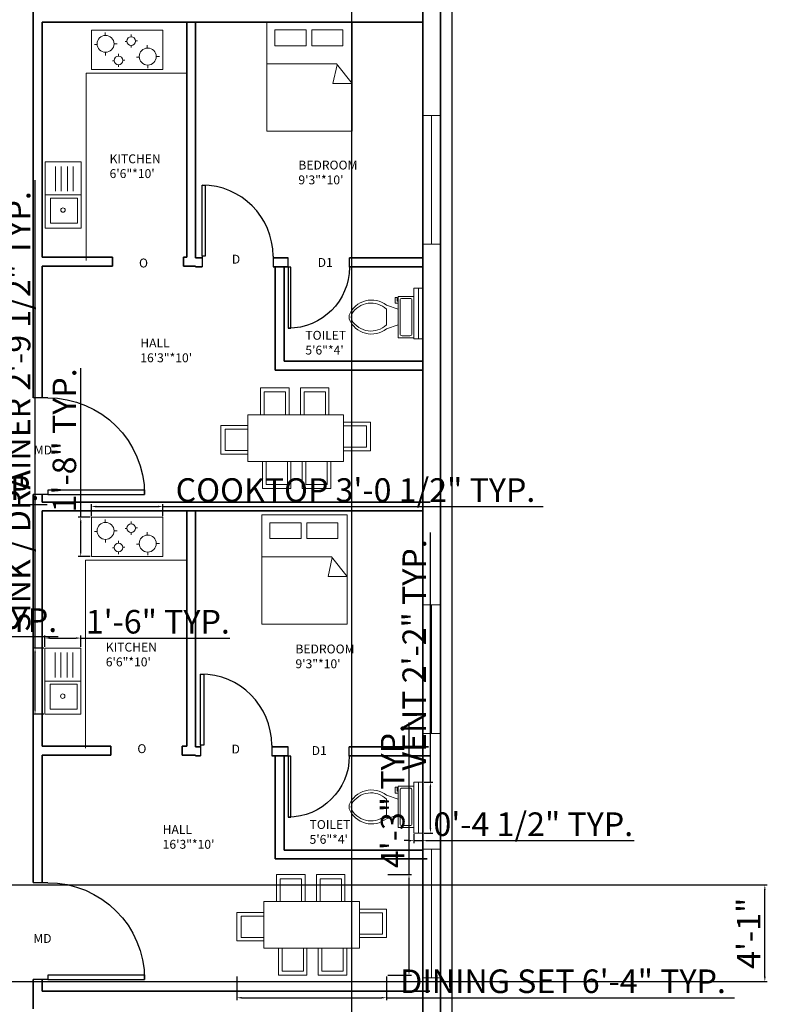
# Model space of a CAD drawing. Units: inches. Extents: x 1947 to 2903, y 1974 to 3472.
# Tile 4 of 5: x 2523 to 2903, y 2335 to 2836. Entities that reach past the tile are written whole.
import ezdxf

# ---------------------------------------------------------------- set-up
doc = ezdxf.new("R2010")
doc.units = ezdxf.units.IN
for name, color, linetype, lineweight in [('A-ANNO-DIMS', 2, 'Continuous', 18), ('A-ANNO-TEXT', 7, 'Continuous', 18), ('A-AREA-IDEN', 7, 'Continuous', 18), ('A-DOOR', 3, 'Continuous', 25), ('A-EQPM', 8, 'Continuous', 18), ('A-FLOR-CASE', 8, 'Continuous', 18), ('A-FLOR-FIXT', 9, 'Continuous', 18), ('A-FURN', 8, 'Continuous', 18), ('A-GLAZ', 4, 'Continuous', 18), ('A-GLAZ-VENT', 4, 'Continuous', 18), ('A-WALL', 7, 'Continuous', 35), ('C-PROP', 1, 'Continuous', 25)]:
    doc.layers.add(name, color=color, linetype=linetype, lineweight=lineweight)
doc.styles.get("Standard").update_dxf_attribs({"font": 'arial.ttf'})
doc.dimstyles.new('ISO-25', dxfattribs={"dimtxt": 12, "dimasz": 2.5, "dimexe": 1.25, "dimexo": 0.625, "dimtad": 1, "dimdec": 0, "dimlunit": 4, "dimtxsty": 'Standard', "dimcen": 2.5, "dimadec": 0, "dimazin": 0, "dimtfac": 1, "dimtdec": 0, "dimtmove": 0, "dimatfit": 3, "dimfxl": 1, "dimarcsym": 0})

# ---------------------------------------------------------------- blocks, each defined once
blk = doc.blocks.new('*U2')
for p, q in [((0, 0), (0, -6)), ((40, 0), (40, -6))]:
    blk.add_line(p, q)
blk.add_lwpolyline([(0, 0), (0, 40), (1.75, 40), (1.75, 0)], close=True)
blk.add_arc((0, 0), 40, 0, 90)
blk = doc.blocks.new('*U4')
for p, q in [((9.5, -6), (9.5, -2)), ((-10, -8.5), (-8, -8.5)), ((-10, -9.5), (-10, -8.5)), ((-7, -9.5), (-10, -9.5)), ((-8, -8.5), (-8, -8)), ((-7, -8), (-7, -9.5)), ((-4, -8), (-6, -14)), ((4, -8), (6, -14)), ((4, -14), (-4, -14))]:
    blk.add_line(p, q)
blk.add_lwpolyline([(10.5, -8), (10.5, 0), (-10.5, 0), (-10.5, -8)], close=True)
for points in [[(-9.5, -2), (-9.5, -6)], [(8.5, -1), (-8.5, -1)], [(-8.5, -7), (8.5, -7)]]:
    blk.add_lwpolyline(points)
for centre, radius, start, end in [((-8.62, -1.88), 0.884, 81.8699, 188.1301), ((8.62, -1.88), 0.884, 351.8699, 98.1301), ((-8.62, -6.12), 0.884, 171.8699, 278.1301), ((8.62, -6.12), 0.884, 261.8699, 8.1301), ((3.52, -21.58), 12.17, 141.4691, 247.9714), ((4.2, -21.82), 11.33, 136.3677, 238.9468), ((-3.52, -21.58), 12.17, 292.0284, 38.5307), ((-4.2, -21.82), 11.33, 301.053, 43.6321), ((0, -27.88), 4, 245.7318, 294.2682), ((0, -29), 4, 254.8605, 285.1395)]:
    blk.add_arc(centre, radius, start, end)
blk = doc.blocks.new('BED-TWO-PILLOWS')
for p, q in [((0, 34.29), (35.37, 34.29)), ((33.59, 24.29), (35.7, 33.87)), ((35.37, 34.29), (43.32, 24.29)), ((43.32, 24.29), (33.59, 24.29))]:
    blk.add_line(p, q)
for points in [[(0, 55.57), (43.32, 55.57), (43.32, 0), (0, 0)], [(4.07, 51.54), (19.88, 51.54), (19.88, 43.48), (4.07, 43.48)], [(22.78, 51.54), (38.59, 51.54), (38.59, 43.48), (22.78, 43.48)]]:
    blk.add_lwpolyline(points, close=True)
blk = doc.blocks.new('DINING-SET-6')
for p, q in [((20.16, 37.5), (20.16, 51.24)), ((20.16, 51.24), (34.7, 51.24)), ((34.7, 51.24), (34.7, 37.5)), ((40.4, 37.5), (40.4, 51.24)), ((40.4, 51.24), (54.94, 51.24)), ((54.94, 51.24), (54.94, 37.5)), ((13.74, 31.99), (0, 31.99)), ((0, 31.99), (0, 17.45)), ((62.33, 33.71), (76.07, 33.71)), ((76.07, 33.71), (76.07, 19.17)), ((0, 17.45), (13.74, 17.45)), ((76.07, 19.17), (62.33, 19.17)), ((21.08, 13.74), (21.08, 0)), ((35.62, 0), (35.62, 13.74)), ((41.32, 13.74), (41.32, 0)), ((55.86, 0), (55.86, 13.74)), ((21.08, 0), (35.62, 0)), ((41.32, 0), (55.86, 0))]:
    blk.add_line(p, q)
for points in [[(22.02, 37.5), (32.87, 37.5), (32.87, 49.12), (22.02, 49.12)], [(42.26, 37.5), (53.11, 37.5), (53.11, 49.12), (42.26, 49.12)], [(13.74, 13.74), (62.33, 13.74), (62.33, 37.5), (13.74, 37.5)], [(13.74, 30.13), (13.74, 19.28), (2.12, 19.28), (2.12, 30.13)], [(62.33, 31.85), (62.33, 21), (73.95, 21), (73.95, 31.85)], [(22.94, 13.74), (33.79, 13.74), (33.79, 2.12), (22.94, 2.12)], [(43.18, 13.74), (54.03, 13.74), (54.03, 2.12), (43.18, 2.12)]]:
    blk.add_lwpolyline(points, close=True)
blk = doc.blocks.new('COOKTOP-4-BURNER')
for p, q in [((6.9, 17.32), (6.9, 18.83)), ((20.11, 16.62), (20.11, 17.76)), ((2.85, 12.63), (1.48, 12.63)), ((11.47, 13.09), (13.05, 13.09)), ((17.95, 14.27), (17.07, 14.27)), ((20.18, 12.22), (20.18, 11.07)), ((22.35, 14.5), (23.33, 14.5)), ((28.35, 10.88), (28.35, 12.39)), ((7.15, 8.69), (7.15, 7.15)), ((13.68, 6.8), (13.68, 7.94)), ((24.3, 6.18), (22.93, 6.18)), ((32.92, 6.64), (34.51, 6.64)), ((11.52, 4.44), (10.65, 4.44)), ((13.75, 2.39), (13.75, 1.25)), ((15.92, 4.68), (16.91, 4.68)), ((28.6, 2.24), (28.6, 0.7))]:
    blk.add_line(p, q)
blk.add_lwpolyline([(0, 0), (36.35, 0), (36.35, 19.93), (0, 19.93)], close=True)
for centre, radius in [((7.15, 13.01), 4.32), ((20.14, 14.42), 2.2), ((28.6, 6.56), 4.32), ((13.72, 4.6), 2.2)]:
    blk.add_circle(centre, radius)
blk = doc.blocks.new('SINK-DRAINER-4')
for p, q in [((5.19, 18.66), (5.19, 31.31)), ((8.1, 18.66), (8.1, 31.31)), ((11.22, 18.66), (11.22, 31.31)), ((14.13, 18.66), (14.13, 31.31)), ((0, 16.81), (18.23, 16.81))]:
    blk.add_line(p, q)
for points in [[(0, 0), (18.23, 0), (18.23, 33.61), (0, 33.61)], [(2.68, 15.14), (16.44, 15.14), (16.44, 2.49), (2.68, 2.49)]]:
    blk.add_lwpolyline(points, close=True)
blk.add_circle((9.01, 9.12), 1.11)
blk = doc.blocks.new('WINDOW-EXTERIOR')
blk.add_line((0, 4.5), (65.51, 4.5))
blk.add_lwpolyline([(0, 0), (65.51, 0), (65.51, 9), (0, 9)], close=True)
blk = doc.blocks.new('VENT-TOILET')
blk.add_line((2.25, 0), (2.25, 25.89))
blk.add_lwpolyline([(0, 25.89), (4.5, 25.89), (4.5, 0), (0, 0)], close=True)
blk = doc.blocks.new('*D20')
at = {"layer": 'A-ANNO-DIMS', "color": 0, "lineweight": -2, "transparency": 16777216}
for p, q in [((2394.54, 2530.2), (2394.54, 2521.24)), ((2437.85, 2530.2), (2437.85, 2521.24)), ((2397.04, 2522.49), (2435.35, 2522.49)), ((2437.85, 2522.49), (2542.7, 2522.49))]:
    blk.add_line(p, q, dxfattribs=at)
at = {"layer": 'A-ANNO-DIMS', "color": 0, "lineweight": 100, "transparency": 16777216}
for points in [[(2397.04, 2522.91), (2397.04, 2522.07), (2394.54, 2522.49)], [(2435.35, 2522.91), (2435.35, 2522.07), (2437.85, 2522.49)]]:
    blk.add_solid(points, dxfattribs=at)
at = {"layer": 'Defpoints', "color": 0, "lineweight": 100, "transparency": 16777216}
for p in [(2394.54, 2530.83), (2437.85, 2530.83), (2437.85, 2522.49)]:
    blk.add_point(p, dxfattribs=at)
at = {"layer": 'A-ANNO-DIMS', "color": 0, "transparency": 16777216, "insert": (2491.53, 2529.32), "char_height": 12, "attachment_point": 5}
blk.add_mtext('3\'-7 1/2" TYP.', dxfattribs=at)
blk = doc.blocks.new('*D21')
at = {"layer": 'A-ANNO-DIMS', "color": 0, "lineweight": -2, "transparency": 16777216}
for p, q in [((2633.63, 2349.59), (2633.63, 2337.56)), ((2709.7, 2349.59), (2709.7, 2337.56)), ((2636.13, 2338.81), (2707.2, 2338.81)), ((2709.7, 2338.81), (2886.59, 2338.81))]:
    blk.add_line(p, q, dxfattribs=at)
at = {"layer": 'A-ANNO-DIMS', "color": 0, "lineweight": 100, "transparency": 16777216}
for points in [[(2636.13, 2339.22), (2636.13, 2338.39), (2633.63, 2338.81)], [(2707.2, 2339.22), (2707.2, 2338.39), (2709.7, 2338.81)]]:
    blk.add_solid(points, dxfattribs=at)
at = {"layer": 'Defpoints', "color": 0, "lineweight": 100, "transparency": 16777216}
for p in [(2633.63, 2350.22), (2709.7, 2350.22), (2709.7, 2338.81)]:
    blk.add_point(p, dxfattribs=at)
at = {"layer": 'A-ANNO-DIMS', "color": 0, "transparency": 16777216, "insert": (2799.39, 2345.64), "char_height": 12, "attachment_point": 5}
blk.add_mtext('DINING SET 6\'-4" TYP.', dxfattribs=at)
blk = doc.blocks.new('*D22')
at = {"layer": 'A-ANNO-DIMS', "color": 0, "lineweight": -2, "transparency": 16777216}
for p, q in [((2721.11, 2401.45), (2721.11, 2478.83)), ((2710.32, 2401.45), (2722.36, 2401.45)), ((2721.11, 2352.72), (2721.11, 2398.95)), ((2710.32, 2350.22), (2722.36, 2350.22))]:
    blk.add_line(p, q, dxfattribs=at)
at = {"layer": 'A-ANNO-DIMS', "color": 0, "lineweight": 100, "transparency": 16777216}
for points in [[(2720.69, 2398.95), (2721.52, 2398.95), (2721.11, 2401.45)], [(2720.69, 2352.72), (2721.52, 2352.72), (2721.11, 2350.22)]]:
    blk.add_solid(points, dxfattribs=at)
at = {"layer": 'Defpoints', "color": 0, "lineweight": 100, "transparency": 16777216}
for p in [(2709.7, 2401.45), (2721.11, 2401.45), (2709.7, 2350.22)]:
    blk.add_point(p, dxfattribs=at)
at = {"layer": 'A-ANNO-DIMS', "color": 0, "transparency": 16777216, "insert": (2714.35, 2441.39), "char_height": 12, "attachment_point": 5, "rotation": 90}
blk.add_mtext('4\'-3" TYP.', dxfattribs=at)
blk = doc.blocks.new('*D23')
at = {"layer": 'A-ANNO-DIMS', "color": 0, "lineweight": -2, "transparency": 16777216}
for p, q in [((2731.99, 2448.48), (2731.99, 2575.36)), ((2728.74, 2448.48), (2733.24, 2448.48)), ((2731.99, 2425.08), (2731.99, 2445.98)), ((2728.74, 2422.58), (2733.24, 2422.58))]:
    blk.add_line(p, q, dxfattribs=at)
at = {"layer": 'A-ANNO-DIMS', "color": 0, "lineweight": 100, "transparency": 16777216}
for points in [[(2731.58, 2445.98), (2732.41, 2445.98), (2731.99, 2448.48)], [(2731.58, 2425.08), (2732.41, 2425.08), (2731.99, 2422.58)]]:
    blk.add_solid(points, dxfattribs=at)
at = {"layer": 'Defpoints', "color": 0, "lineweight": 100, "transparency": 16777216}
for p in [(2728.11, 2448.48), (2731.99, 2448.48), (2728.11, 2422.58)]:
    blk.add_point(p, dxfattribs=at)
at = {"layer": 'A-ANNO-DIMS', "color": 0, "transparency": 16777216, "insert": (2725.34, 2513.17), "char_height": 12, "attachment_point": 5, "rotation": 90}
blk.add_mtext('VENT 2\'-2" TYP.', dxfattribs=at)
blk = doc.blocks.new('*D24')
at = {"layer": 'A-ANNO-DIMS', "color": 0, "lineweight": -2, "transparency": 16777216}
for p, q in [((2723.61, 2421.96), (2723.61, 2417.45)), ((2728.11, 2421.96), (2728.11, 2417.45)), ((2721.11, 2418.7), (2718.61, 2418.7)), ((2723.61, 2418.7), (2728.11, 2418.7)), ((2730.61, 2418.7), (2835.47, 2418.7))]:
    blk.add_line(p, q, dxfattribs=at)
at = {"layer": 'A-ANNO-DIMS', "color": 0, "lineweight": 100, "transparency": 16777216}
for points in [[(2721.11, 2419.12), (2721.11, 2418.28), (2723.61, 2418.7)], [(2730.61, 2419.12), (2730.61, 2418.28), (2728.11, 2418.7)]]:
    blk.add_solid(points, dxfattribs=at)
at = {"layer": 'Defpoints', "color": 0, "lineweight": 100, "transparency": 16777216}
for p in [(2723.61, 2422.58), (2728.11, 2422.58), (2728.11, 2418.7)]:
    blk.add_point(p, dxfattribs=at)
at = {"layer": 'A-ANNO-DIMS', "color": 0, "transparency": 16777216, "insert": (2784.29, 2425.53), "char_height": 12, "attachment_point": 5}
blk.add_mtext('0\'-4 1/2" TYP.', dxfattribs=at)
blk = doc.blocks.new('*D25')
at = {"layer": 'A-ANNO-DIMS', "color": 0, "lineweight": -2, "transparency": 16777216}
for p, q in [((2559.69, 2583.8), (2559.69, 2589.88)), ((2596.03, 2583.8), (2596.03, 2589.88)), ((2562.19, 2588.63), (2593.53, 2588.63)), ((2596.03, 2588.63), (2789.24, 2588.63))]:
    blk.add_line(p, q, dxfattribs=at)
at = {"layer": 'A-ANNO-DIMS', "color": 0, "lineweight": 100, "transparency": 16777216}
for points in [[(2562.19, 2589.05), (2562.19, 2588.22), (2559.69, 2588.63)], [(2593.53, 2589.05), (2593.53, 2588.22), (2596.03, 2588.63)]]:
    blk.add_solid(points, dxfattribs=at)
at = {"layer": 'Defpoints', "color": 0, "lineweight": 100, "transparency": 16777216}
for p in [(2596.03, 2588.63), (2559.69, 2583.18), (2596.03, 2583.18)]:
    blk.add_point(p, dxfattribs=at)
at = {"layer": 'A-ANNO-DIMS', "color": 0, "transparency": 16777216, "insert": (2693.89, 2595.47), "char_height": 12, "attachment_point": 5}
blk.add_mtext('COOKTOP 3\'-0 1/2" TYP.', dxfattribs=at)
blk = doc.blocks.new('*D26')
at = {"layer": 'A-ANNO-DIMS', "color": 0, "lineweight": -2, "transparency": 16777216}
for p, q in [((2554.23, 2583.18), (2554.23, 2658.95)), ((2559.06, 2583.18), (2552.98, 2583.18)), ((2554.23, 2565.75), (2554.23, 2580.68)), ((2559.06, 2563.25), (2552.98, 2563.25))]:
    blk.add_line(p, q, dxfattribs=at)
at = {"layer": 'A-ANNO-DIMS', "color": 0, "lineweight": 100, "transparency": 16777216}
for points in [[(2553.82, 2580.68), (2554.65, 2580.68), (2554.23, 2583.18)], [(2553.82, 2565.75), (2554.65, 2565.75), (2554.23, 2563.25)]]:
    blk.add_solid(points, dxfattribs=at)
at = {"layer": 'Defpoints', "color": 0, "lineweight": 100, "transparency": 16777216}
for p in [(2554.23, 2583.18), (2559.69, 2583.18), (2559.69, 2563.25)]:
    blk.add_point(p, dxfattribs=at)
at = {"layer": 'A-ANNO-DIMS', "color": 0, "transparency": 16777216, "insert": (2547.48, 2622.31), "char_height": 12, "attachment_point": 5, "rotation": 90}
blk.add_mtext('1\'-8" TYP.', dxfattribs=at)
blk = doc.blocks.new('*D29')
at = {"layer": 'A-ANNO-DIMS', "color": 0, "lineweight": -2, "transparency": 16777216}
for p, q in [((2531.02, 2516.69), (2531.02, 2754.7)), ((2535.44, 2516.69), (2529.77, 2516.69)), ((2531.02, 2485.58), (2531.02, 2514.19)), ((2535.44, 2483.08), (2529.77, 2483.08))]:
    blk.add_line(p, q, dxfattribs=at)
at = {"layer": 'A-ANNO-DIMS', "color": 0, "lineweight": 100, "transparency": 16777216}
for points in [[(2530.61, 2514.19), (2531.44, 2514.19), (2531.02, 2516.69)], [(2530.61, 2485.58), (2531.44, 2485.58), (2531.02, 2483.08)]]:
    blk.add_solid(points, dxfattribs=at)
at = {"layer": 'Defpoints', "color": 0, "lineweight": 100, "transparency": 16777216}
for p in [(2531.02, 2516.69), (2536.07, 2516.69), (2536.07, 2483.08)]:
    blk.add_point(p, dxfattribs=at)
at = {"layer": 'A-ANNO-DIMS', "color": 0, "transparency": 16777216, "insert": (2524.19, 2636.95), "char_height": 12, "attachment_point": 5, "rotation": 90}
blk.add_mtext('SINK / DRAINER 2\'-9 1/2" TYP.', dxfattribs=at)
blk = doc.blocks.new('*D30')
at = {"layer": 'A-ANNO-DIMS', "color": 0, "lineweight": -2, "transparency": 16777216}
for p, q in [((2536.07, 2517.32), (2536.07, 2522.99)), ((2538.57, 2521.74), (2551.8, 2521.74)), ((2554.3, 2517.32), (2554.3, 2522.99)), ((2554.3, 2521.74), (2630.07, 2521.74))]:
    blk.add_line(p, q, dxfattribs=at)
at = {"layer": 'A-ANNO-DIMS', "color": 0, "lineweight": 100, "transparency": 16777216}
for points in [[(2538.57, 2522.15), (2538.57, 2521.32), (2536.07, 2521.74)], [(2551.8, 2522.15), (2551.8, 2521.32), (2554.3, 2521.74)]]:
    blk.add_solid(points, dxfattribs=at)
at = {"layer": 'Defpoints', "color": 0, "lineweight": 100, "transparency": 16777216}
for p in [(2554.3, 2521.74), (2536.07, 2516.69), (2554.3, 2516.69)]:
    blk.add_point(p, dxfattribs=at)
at = {"layer": 'A-ANNO-DIMS', "color": 0, "transparency": 16777216, "insert": (2593.43, 2528.49), "char_height": 12, "attachment_point": 5}
blk.add_mtext('1\'-6" TYP.', dxfattribs=at)
blk = doc.blocks.new('*D31')
at = {"layer": 'A-ANNO-DIMS', "color": 0, "lineweight": -2, "transparency": 16777216}
for p, q in [((2307.69, 2584.79), (2307.69, 2590.86)), ((2310.19, 2589.61), (2341.53, 2589.61)), ((2344.03, 2584.79), (2344.03, 2590.86)), ((2344.03, 2589.61), (2537.24, 2589.61))]:
    blk.add_line(p, q, dxfattribs=at)
at = {"layer": 'A-ANNO-DIMS', "color": 0, "lineweight": 100, "transparency": 16777216}
for points in [[(2310.19, 2590.03), (2310.19, 2589.2), (2307.69, 2589.61)], [(2341.53, 2590.03), (2341.53, 2589.2), (2344.03, 2589.61)]]:
    blk.add_solid(points, dxfattribs=at)
at = {"layer": 'Defpoints', "color": 0, "lineweight": 100, "transparency": 16777216}
for p in [(2344.03, 2589.61), (2307.69, 2584.16), (2344.03, 2584.16)]:
    blk.add_point(p, dxfattribs=at)
at = {"layer": 'A-ANNO-DIMS', "color": 0, "transparency": 16777216, "insert": (2441.89, 2596.45), "char_height": 12, "attachment_point": 5}
blk.add_mtext('COOKTOP 3\'-0 1/2" TYP.', dxfattribs=at)
blk = doc.blocks.new('*D36')
at = {"layer": 'A-ANNO-DIMS', "color": 0, "lineweight": -2, "transparency": 16777216}
for p, q in [((2692.11, 2238.03), (2692.11, 3458.67)), ((2694.61, 3457.42), (2725.61, 3457.42)), ((2728.11, 2238.03), (2728.11, 3458.67))]:
    blk.add_line(p, q, dxfattribs=at)
at = {"layer": 'A-ANNO-DIMS', "color": 0, "lineweight": 100, "transparency": 16777216}
for points in [[(2694.61, 3457.83), (2694.61, 3457), (2692.11, 3457.42)], [(2725.61, 3457.83), (2725.61, 3457), (2728.11, 3457.42)]]:
    blk.add_solid(points, dxfattribs=at)
at = {"layer": 'Defpoints', "color": 0, "lineweight": 100, "transparency": 16777216}
for p in [(2728.11, 3457.42), (2692.11, 2237.41), (2728.11, 2237.41)]:
    blk.add_point(p, dxfattribs=at)
at = {"layer": 'A-ANNO-DIMS', "color": 0, "transparency": 16777216, "insert": (2710.11, 3464.17), "char_height": 12, "attachment_point": 5}
blk.add_mtext('3\'-0"', dxfattribs=at)
blk = doc.blocks.new('*D39')
at = {"layer": 'A-ANNO-DIMS', "color": 0, "lineweight": -2, "transparency": 16777216}
for p, q in [((2476.73, 2396.2), (2903.22, 2396.2)), ((2901.97, 2349.5), (2901.97, 2393.7)), ((2476.73, 2347), (2903.22, 2347))]:
    blk.add_line(p, q, dxfattribs=at)
at = {"layer": 'A-ANNO-DIMS', "color": 0, "lineweight": 100, "transparency": 16777216}
for points in [[(2901.55, 2393.7), (2902.39, 2393.7), (2901.97, 2396.2)], [(2901.55, 2349.5), (2902.39, 2349.5), (2901.97, 2347)]]:
    blk.add_solid(points, dxfattribs=at)
at = {"layer": 'Defpoints', "color": 0, "lineweight": 100, "transparency": 16777216}
for p in [(2476.11, 2396.2), (2901.97, 2396.2), (2476.11, 2347)]:
    blk.add_point(p, dxfattribs=at)
at = {"layer": 'A-ANNO-DIMS', "color": 0, "transparency": 16777216, "insert": (2895.32, 2371.6), "char_height": 12, "attachment_point": 5, "rotation": 90}
blk.add_mtext('4\'-1"', dxfattribs=at)

msp = doc.modelspace()

# ---------------------------------------------------------------- linework, layer by layer
at = {"layer": 'A-FLOR-CASE'}
for p, q in [((2556.95, 2713.82), (2556.95, 2809.13)), ((2608.11, 2809.13), (2556.95, 2809.13)), ((2556.71, 2465.74), (2556.71, 2561.41)), ((2608.11, 2561.41), (2556.71, 2561.41))]:
    msp.add_line(p, q, dxfattribs=at)
at = {"layer": 'A-WALL'}
for p, q in [((2728.11, 2848.84), (2728.11, 2835.06)), ((2530.11, 2843.44), (2530.11, 2643.97)), ((2534.61, 2835.06), (2728.11, 2835.06)), ((2534.61, 2835.06), (2728.11, 2835.06)), ((2534.61, 2835.06), (2534.61, 2715.39)), ((2608.11, 2835.06), (2608.11, 2715.39)), ((2612.61, 2835.06), (2612.61, 2715.06)), ((2612.61, 2835.06), (2723.61, 2835.06)), ((2728.11, 2835.06), (2728.11, 2710.56)), ((2530.11, 2715.39), (2530.11, 2715.39)), ((2570.32, 2715.39), (2534.61, 2715.39)), ((2570.32, 2710.89), (2570.32, 2715.39)), ((2608.11, 2715.39), (2606.46, 2715.39)), ((2606.46, 2710.89), (2606.46, 2715.39)), ((2615.89, 2715.06), (2612.61, 2715.06)), ((2659.74, 2715.06), (2652.03, 2715.06)), ((2723.61, 2715.06), (2690.84, 2715.06)), ((2723.61, 2715.06), (2728.11, 2715.06)), ((2530.11, 2710.89), (2530.11, 2710.89)), ((2570.32, 2710.89), (2534.61, 2710.89)), ((2534.61, 2710.89), (2534.61, 2643.97)), ((2612.61, 2710.89), (2606.46, 2710.89)), ((2615.89, 2710.56), (2612.61, 2710.56)), ((2659.74, 2710.56), (2652.03, 2710.56)), ((2653.11, 2658.06), (2653.11, 2710.56)), ((2657.61, 2662.56), (2657.61, 2710.56)), ((2723.61, 2710.56), (2690.84, 2710.56)), ((2723.61, 2710.56), (2728.11, 2710.56)), ((2728.11, 2711.09), (2728.11, 2591.09)), ((2728.11, 2710.56), (2728.11, 2644.87)), ((2737.11, 2713.55), (2737.11, 2593.55)), ((2723.61, 2662.56), (2657.61, 2662.56)), ((2723.61, 2662.56), (2728.11, 2662.56)), ((2723.61, 2658.06), (2653.11, 2658.06)), ((2723.18, 2658.06), (2728.11, 2658.06)), ((2530.11, 2594.77), (2530.11, 2397.34)), ((2534.61, 2594.77), (2534.61, 2590.89)), ((2728.11, 2595.67), (2728.11, 2586.39)), ((2728.11, 2595.67), (2728.11, 2586.39)), ((2534.61, 2590.89), (2723.61, 2590.89)), ((2534.61, 2590.89), (2723.61, 2590.89)), ((2723.3, 2590.89), (2731.88, 2590.89)), ((2534.61, 2586.39), (2728.11, 2586.39)), ((2534.61, 2586.39), (2728.11, 2586.39)), ((2534.61, 2586.39), (2534.61, 2466.72)), ((2608.11, 2586.39), (2608.11, 2466.72)), ((2612.61, 2586.39), (2612.61, 2466.39)), ((2612.61, 2586.39), (2723.61, 2586.39)), ((2728.11, 2586.39), (2728.11, 2461.89)), ((2530.11, 2466.72), (2530.11, 2466.72)), ((2569.62, 2466.72), (2534.61, 2466.72)), ((2569.62, 2462.22), (2569.62, 2466.72)), ((2608.11, 2466.72), (2605.75, 2466.72)), ((2605.75, 2462.22), (2605.75, 2466.72)), ((2615.18, 2466.39), (2612.61, 2466.39)), ((2659.63, 2466.39), (2651.32, 2466.39)), ((2723.61, 2466.39), (2690.73, 2466.39)), ((2723.61, 2466.39), (2731.05, 2466.39)), ((2737.11, 2464.88), (2737.11, 2344.88)), ((2530.11, 2462.22), (2530.11, 2462.22)), ((2569.62, 2462.22), (2534.61, 2462.22)), ((2534.61, 2462.22), (2534.61, 2397.34)), ((2612.61, 2462.22), (2605.75, 2462.22)), ((2615.18, 2461.89), (2612.61, 2461.89)), ((2659.63, 2461.89), (2651.32, 2461.89)), ((2653.11, 2409.39), (2653.11, 2461.89)), ((2657.61, 2413.89), (2657.61, 2461.89)), ((2723.61, 2461.89), (2690.73, 2461.89)), ((2723.61, 2461.89), (2731.66, 2461.89)), ((2728.11, 2462.41), (2728.11, 2342.41)), ((2728.11, 2461.89), (2728.11, 2395.75)), ((2723.61, 2413.89), (2657.61, 2413.89)), ((2723.61, 2413.89), (2728.34, 2413.89)), ((2723.61, 2409.39), (2653.11, 2409.39)), ((2723.61, 2409.39), (2730.27, 2409.39)), ((2530.11, 2348.13), (2530.11, 2333.22)), ((2534.61, 2348.13), (2534.61, 2342.22)), ((2728.11, 2347), (2728.11, 2333.22)), ((2728.11, 2347), (2728.11, 2337.72)), ((2534.61, 2342.22), (2723.61, 2342.22)), ((2723.61, 2342.22), (2731.66, 2342.22))]:
    msp.add_line(p, q, dxfattribs=at)
for points in [[(2269.11, 2228.41), (2737.11, 2228.41), (2737.11, 3341.41), (2269.11, 3341.41)], [(2278.11, 2237.41), (2728.11, 2237.41), (2728.11, 3332.41), (2278.11, 3332.41)]]:
    msp.add_lwpolyline(points, close=True, dxfattribs=at)
at = {"layer": 'C-PROP'}
msp.add_line((2743.11, 2228.41), (2743.11, 3341.41), dxfattribs=at)

# ---------------------------------------------------------------- block references
at = {"layer": 'A-DOOR', "xscale": 0.9034599273514711, "yscale": 0.9034599273514711, "zscale": 0.9034599273514711}
for p in [(2615.89, 2715.98), (2615.18, 2467.31)]:
    msp.add_blockref('*U2', p, dxfattribs=at)
at = {"layer": 'A-DOOR'}
for p, xscale, yscale, zscale, rotation in [((2659.74, 2710.4), -0.7774936004188162, 0.7774936004188162, 0.7774936004188162, 180), ((2537.49, 2594.77), -1.23010588698369, 1.23010588698369, 1.23010588698369, 270), ((2659.63, 2461.73), -0.7774936004188162, 0.7774936004188162, 0.7774936004188162, 180), ((2537.49, 2348.13), -1.23010588698369, 1.23010588698369, 1.23010588698369, 270)]:
    msp.add_blockref('*U2', p, dxfattribs=dict(at, xscale=xscale, yscale=yscale, zscale=zscale, rotation=rotation))
at = {"layer": 'A-EQPM'}
for p in [(2559.69, 2810.97), (2559.69, 2563.25)]:
    msp.add_blockref('COOKTOP-4-BURNER', p, dxfattribs=at)
at = {"layer": 'A-FLOR-FIXT'}
for p in [(2536.22, 2730.3), (2536.07, 2483.08)]:
    msp.add_blockref('SINK-DRAINER-4', p, dxfattribs=at)
at = {"layer": 'A-FLOR-FIXT', "rotation": 270}
for p in [(2723.61, 2685.01), (2723.61, 2435.87)]:
    msp.add_blockref('*U4', p, dxfattribs=at)
at = {"layer": 'A-FURN'}
for name, p in [('BED-TWO-PILLOWS', (2648.88, 2779.5)), ('DINING-SET-6', (2625.49, 2597.79)), ('BED-TWO-PILLOWS', (2646.38, 2528.84)), ('DINING-SET-6', (2633.63, 2350.22))]:
    msp.add_blockref(name, p, dxfattribs=at)
at = {"layer": 'A-GLAZ'}
for p, rotation in [((2728.11, 2787.57), 269.9999999999988), ((2728.11, 2538.65), 269.9999999999986), ((2728.11, 2414.41), 269.9999999999986)]:
    msp.add_blockref('WINDOW-EXTERIOR', p, dxfattribs=dict(at, rotation=rotation))
at = {"layer": 'A-GLAZ-VENT'}
for p in [(2723.61, 2673.9), (2723.61, 2422.58)]:
    msp.add_blockref('VENT-TOILET', p, dxfattribs=at)

# ---------------------------------------------------------------- texts
at = {"layer": 'A-ANNO-TEXT', "attachment_point": 1}
for s, insert, char_height in [('O', (2583.87, 2714.76), 4.52), ('D', (2631.05, 2716.71), 4.52), ('D1', (2674.7, 2715.04), 4.519), ('MD', (2530.43, 2619.63), 4.519), ('O', (2583.04, 2467.74), 4.52), ('D', (2630.91, 2467.56), 4.52), ('D1', (2671.64, 2466.77), 4.519), ('MD', (2530.17, 2371.22), 4.519)]:
    msp.add_mtext_dynamic_manual_height_columns(s, width=35.9327, gutter_width=22.59, heights=[0], dxfattribs=dict(at, insert=insert, char_height=char_height))
at = {"layer": 'A-AREA-IDEN', "char_height": 4.519, "attachment_point": 1}
for s, insert in [('KITCHEN\\P6\'6"*10\'', (2568.91, 2767.77)), ('BEDROOM\\P9\'3"*10\'', (2664.88, 2764.57)), ('TOILET\\P5\'6"*4\'', (2668.42, 2677.99)), ('HALL\\P16\'3"*10\'', (2584.52, 2674.08)), ('KITCHEN\\P6\'6"*10\'', (2566.99, 2519.4)), ('BEDROOM\\P9\'3"*10\'', (2663.4, 2518.45)), ('TOILET\\P5\'6"*4\'', (2670.56, 2429.16)), ('HALL\\P16\'3"*10\'', (2595.89, 2426.64))]:
    msp.add_mtext_dynamic_manual_height_columns(s, width=35.9327, gutter_width=22.59, heights=[0], dxfattribs=dict(at, insert=insert))

# ---------------------------------------------------------------- dimensions: what is measured, and where the dimension line sits
at = {"layer": 'A-ANNO-DIMS'}
dim = msp.add_linear_dim(base=(2728.11, 3457.42), p1=(2692.11, 2237.41), p2=(2728.11, 2237.41), dimstyle='ISO-25', override={"dimdec": 1, "dimlfac": 1, "dimrnd": 0, "dimzin": 1, "dimdsep": 46, "dimlunit": 4, "dimfrac": 2}, dxfattribs=at)
dim.commit()
dim.dimension.update_dxf_attribs({"geometry": '*D36', "text_midpoint": (2710.11, 3464.17)})
for base, p1, p2, text, picture, middle in [((2531.02, 2516.69), (2536.07, 2483.08), (2536.07, 2516.69), 'SINK / DRAINER <> TYP.', '*D29', (2524.19, 2636.95)), ((2554.23, 2583.18), (2559.69, 2563.25), (2559.69, 2583.18), '<> TYP.', '*D26', (2547.48, 2622.31)), ((2731.99, 2448.48), (2728.11, 2422.58), (2728.11, 2448.48), 'VENT <> TYP.', '*D23', (2725.34, 2513.17)), ((2721.11, 2401.45), (2709.7, 2350.22), (2709.7, 2401.45), '<> TYP.', '*D22', (2714.35, 2441.39))]:
    dim = msp.add_linear_dim(base=base, p1=p1, p2=p2, angle=90, text=text, dimstyle='ISO-25', override={"dimdec": 1, "dimlfac": 1, "dimrnd": 0, "dimzin": 1, "dimdsep": 46, "dimlunit": 4, "dimfrac": 2}, dxfattribs=at)
    dim.commit()
    dim.dimension.update_dxf_attribs({"geometry": picture, "text_midpoint": middle})
for base, p1, p2, text, picture, middle in [((2344.03, 2589.61), (2307.69, 2584.16), (2344.03, 2584.16), 'COOKTOP <> TYP.', '*D31', (2441.89, 2596.45)), ((2596.03, 2588.63), (2559.69, 2583.18), (2596.03, 2583.18), 'COOKTOP <> TYP.', '*D25', (2693.89, 2595.47)), ((2437.85, 2522.49), (2394.54, 2530.83), (2437.85, 2530.83), '<> TYP.', '*D20', (2491.53, 2529.32)), ((2554.3, 2521.74), (2536.07, 2516.69), (2554.3, 2516.69), '<> TYP.', '*D30', (2593.43, 2528.49)), ((2728.11, 2418.7), (2723.61, 2422.58), (2728.11, 2422.58), '<> TYP.', '*D24', (2784.29, 2425.53)), ((2709.7, 2338.81), (2633.63, 2350.22), (2709.7, 2350.22), 'DINING SET <> TYP.', '*D21', (2799.39, 2345.64))]:
    dim = msp.add_linear_dim(base=base, p1=p1, p2=p2, text=text, dimstyle='ISO-25', override={"dimdec": 1, "dimlfac": 1, "dimrnd": 0, "dimzin": 1, "dimdsep": 46, "dimlunit": 4, "dimfrac": 2}, dxfattribs=at)
    dim.commit()
    dim.dimension.update_dxf_attribs({"geometry": picture, "text_midpoint": middle})
dim = msp.add_linear_dim(base=(2901.97, 2396.2), p1=(2476.11, 2347), p2=(2476.11, 2396.2), angle=90, dimstyle='ISO-25', override={"dimdec": 1, "dimlfac": 1, "dimrnd": 0, "dimzin": 1, "dimdsep": 46, "dimlunit": 4, "dimfrac": 2}, dxfattribs=at)
dim.commit()
dim.dimension.update_dxf_attribs({"geometry": '*D39', "text_midpoint": (2895.32, 2371.6)})

doc.saveas('drawing.dxf')
